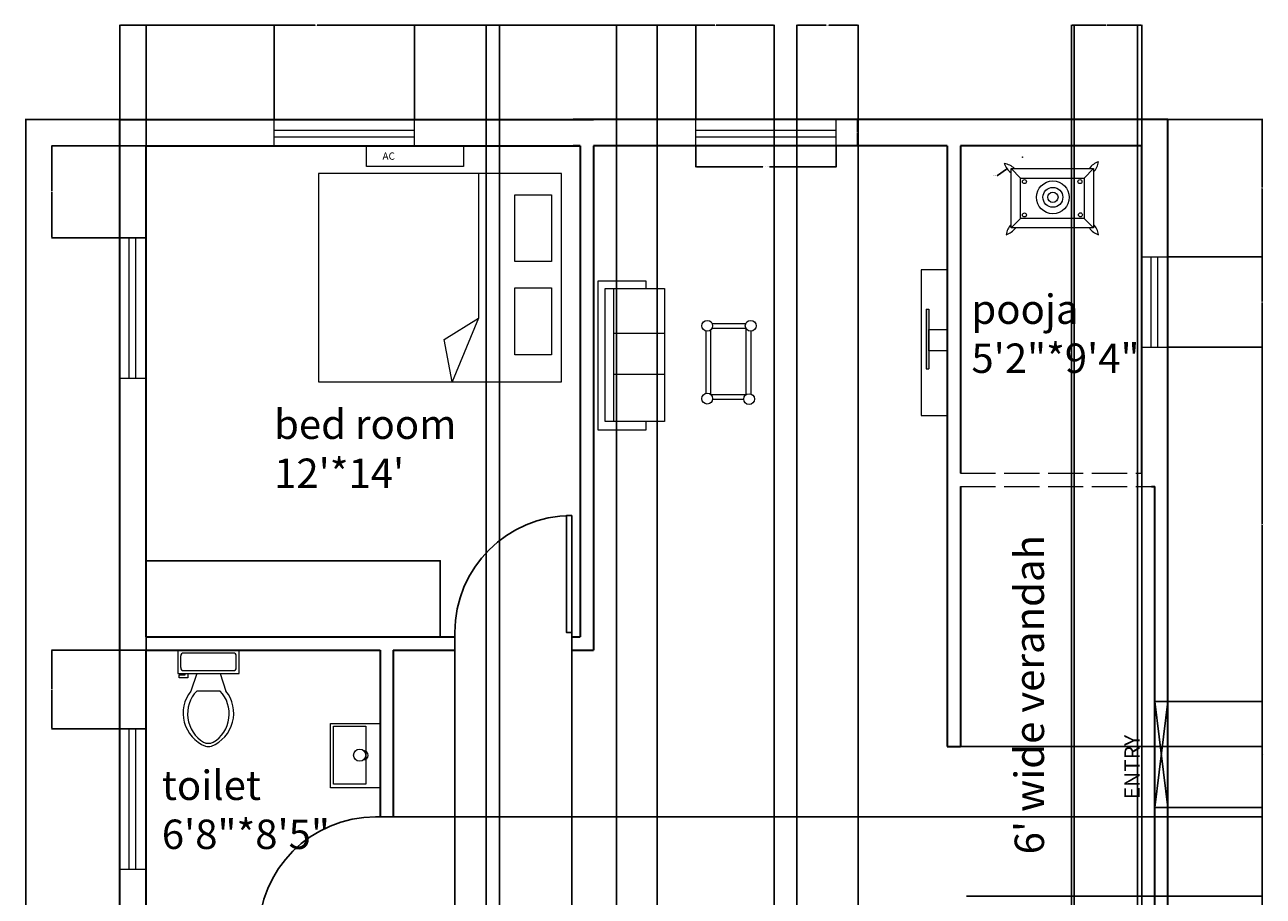
# Model space of a CAD drawing. Units: inches. Extents: x 2187 to 2611, y 763 to 1433.
# Tile 3 of 3: x 2187 to 2611, y 1135 to 1433. Entities that reach past the tile are written whole.
import ezdxf

# ---------------------------------------------------------------- set-up
doc = ezdxf.new("R2010")
doc.units = ezdxf.units.IN
doc.linetypes.add('ACAD_ISO02W100', pattern=[15, 12, -3])
for name, color, linetype, lineweight in [('A-ANNO-DIMS', 2, 'Continuous', 18), ('A-ANNO-TEXT', 7, 'Continuous', 18), ('A-AREA-IDEN', 7, 'Continuous', 18), ('A-FLOR-CASE', 82, 'Continuous', 25), ('A-FLOR-FIXT', 82, 'Continuous', 18), ('A-FURN-PATT', 82, 'Continuous', 13), ('A-WALL', 7, 'Continuous', 35), ('A-WALL-OVHD', 7, 'ACAD_ISO02W100', 18), ('DOOR', 130, 'Continuous', 25), ('FURNITURE', 82, 'Continuous', 18), ('M-HVAC-EQPM', 82, 'Continuous', 18), ('WINDOW', 50, 'Continuous', 20)]:
    doc.layers.add(name, color=color, linetype=linetype, lineweight=lineweight)
doc.styles.get("Standard").update_dxf_attribs({"font": 'arial.ttf'})
doc.dimstyles.get("Standard").update_dxf_attribs({"dimtxt": 0.18, "dimasz": 0.18, "dimexe": 0.18, "dimexo": 0.0625, "dimgap": 0.09, "dimtad": 0, "dimtih": 1, "dimtoh": 1, "dimdec": 4, "dimzin": 0, "dimdsep": 46, "dimtxsty": 'Standard', "dimcen": 0.09, "dimadec": 0, "dimazin": 0, "dimtfac": 1, "dimtdec": 4, "dimtofl": 0, "dimtmove": 0, "dimatfit": 3, "dimfxl": 1, "dimtolj": 1, "dimtzin": 0, "dimarcsym": 0})

# ---------------------------------------------------------------- blocks, each defined once
blk = doc.blocks.new('*U2')
for p, q in [((0, 0), (0, -6)), ((40, 0), (40, -6))]:
    blk.add_line(p, q)
blk.add_lwpolyline([(0, 0), (0, 40), (1.75, 40), (1.75, 0)], close=True)
blk.add_arc((0, 0), 40, 0, 90)
blk = doc.blocks.new('*U4')
for p, q in [((9.5, -6), (9.5, -2)), ((-8, -8.5), (-8, -8)), ((-7, -8), (-7, -9.5)), ((-4, -8), (-6, -14)), ((4, -8), (6, -14)), ((-10, -8.5), (-8, -8.5)), ((-10, -9.5), (-10, -8.5)), ((-7, -9.5), (-10, -9.5)), ((4, -14), (-4, -14))]:
    blk.add_line(p, q)
blk.add_lwpolyline([(10.5, -8), (10.5, 0), (-10.5, 0), (-10.5, -8)], close=True)
for points in [[(-9.5, -2), (-9.5, -6)], [(8.5, -1), (-8.5, -1)], [(-8.5, -7), (8.5, -7)]]:
    blk.add_lwpolyline(points)
for centre, radius, start, end in [((-8.62, -1.88), 0.884, 81.8699, 188.1301), ((8.62, -1.88), 0.884, 351.8699, 98.1301), ((-8.62, -6.12), 0.884, 171.8699, 278.1301), ((8.62, -6.12), 0.884, 261.8699, 8.1301), ((3.52, -21.58), 12.17, 141.4691, 247.9714), ((4.2, -21.82), 11.33, 136.3677, 238.9468), ((-3.52, -21.58), 12.17, 292.0284, 38.5307), ((-4.2, -21.82), 11.33, 301.053, 43.6321), ((0, -27.88), 4, 245.7318, 294.2682), ((0, -29), 4, 254.8605, 285.1395)]:
    blk.add_arc(centre, radius, start, end)
blk = doc.blocks.new('BED-DOUBLE')
for p, q in [((54.72, 71.29), (54.72, 21.8)), ((42.94, 14.53), (54.72, 21.8)), ((54.72, 21.8), (45.71, 0)), ((45.71, 0), (42.94, 14.53))]:
    blk.add_line(p, q)
for points in [[(83.12, 71.29), (0, 71.29), (0, 0), (83.12, 0)], [(67.19, 64.02), (79.65, 64.02), (79.65, 41.18), (67.19, 41.18)], [(67.19, 32.18), (79.65, 32.18), (79.65, 9.34), (67.19, 9.34)]]:
    blk.add_lwpolyline(points, close=True)
blk = doc.blocks.new('WIN-48IN')
for p, q in [((0, 0), (0, 9)), ((48, 0), (48, 9)), ((0, 5.37), (48, 5.37)), ((0, 3.09), (48, 3.09))]:
    blk.add_line(p, q)
blk = doc.blocks.new('*D8')
at = {"layer": 'A-ANNO-DIMS', "color": 0, "lineweight": -2, "transparency": 16777216}
for p, q in [((2416.82, 1391.9), (2416.82, 1384.58)), ((2464.82, 1391.9), (2464.82, 1384.58)), ((2417, 1384.76), (2439.7, 1384.76)), ((2464.64, 1384.76), (2441.94, 1384.76))]:
    blk.add_line(p, q, dxfattribs=at)
at = {"layer": 'A-ANNO-DIMS', "color": 0, "lineweight": 100, "transparency": 16777216}
for points in [[(2417, 1384.79), (2417, 1384.73), (2416.82, 1384.76)], [(2464.64, 1384.79), (2464.64, 1384.73), (2464.82, 1384.76)]]:
    blk.add_solid(points, dxfattribs=at)
at = {"layer": 'Defpoints', "color": 0, "lineweight": 100, "transparency": 16777216}
for p in [(2416.82, 1391.96), (2464.82, 1391.96), (2464.82, 1384.76)]:
    blk.add_point(p, dxfattribs=at)
at = {"layer": 'A-ANNO-DIMS', "color": 0, "transparency": 16777216, "insert": (2440.82, 1384.76), "char_height": 0.18, "attachment_point": 5}
blk.add_mtext('\\A1;WINDOW 48 TYP.', dxfattribs=at)
blk = doc.blocks.new('*D9')
at = {"layer": 'A-ANNO-DIMS', "color": 0, "lineweight": -2, "transparency": 16777216}
for p, q in [((2464.88, 1400.96), (2472.2, 1400.96)), ((2472.02, 1400.78), (2472.02, 1396.64)), ((2472.02, 1392.14), (2472.02, 1396.28)), ((2464.88, 1391.96), (2472.2, 1391.96))]:
    blk.add_line(p, q, dxfattribs=at)
at = {"layer": 'A-ANNO-DIMS', "color": 0, "lineweight": 100, "transparency": 16777216}
for points in [[(2471.99, 1400.78), (2472.05, 1400.78), (2472.02, 1400.96)], [(2471.99, 1392.14), (2472.05, 1392.14), (2472.02, 1391.96)]]:
    blk.add_solid(points, dxfattribs=at)
at = {"layer": 'Defpoints', "color": 0, "lineweight": 100, "transparency": 16777216}
for p in [(2464.82, 1400.96), (2472.02, 1400.96), (2464.82, 1391.96)]:
    blk.add_point(p, dxfattribs=at)
at = {"layer": 'A-ANNO-DIMS', "color": 0, "transparency": 16777216, "insert": (2472.02, 1396.46), "char_height": 0.18, "attachment_point": 5}
blk.add_mtext('\\A1;9 TYP.', dxfattribs=at)
blk = doc.blocks.new('*D15')
at = {"layer": 'A-ANNO-DIMS', "color": 0, "lineweight": -2, "transparency": 16777216}
for p, q in [((2219.71, 1400.96), (2187.39, 1400.96)), ((2187.57, 1400.78), (2187.57, 1120.06)), ((2187.57, 838.97), (2187.57, 1119.7)), ((2219.71, 838.79), (2187.39, 838.79))]:
    blk.add_line(p, q, dxfattribs=at)
at = {"layer": 'A-ANNO-DIMS', "color": 0, "lineweight": 100, "transparency": 16777216}
for points in [[(2187.54, 1400.78), (2187.6, 1400.78), (2187.57, 1400.96)], [(2187.54, 838.97), (2187.6, 838.97), (2187.57, 838.79)]]:
    blk.add_solid(points, dxfattribs=at)
at = {"layer": 'Defpoints', "color": 0, "lineweight": 100, "transparency": 16777216}
for p in [(2187.57, 1400.96), (2219.77, 1400.96), (2219.77, 838.79)]:
    blk.add_point(p, dxfattribs=at)
at = {"layer": 'A-ANNO-DIMS', "color": 0, "transparency": 16777216, "insert": (2187.57, 1119.88), "char_height": 0.18, "attachment_point": 5}
blk.add_mtext('\\A1;562.2', dxfattribs=at)
blk = doc.blocks.new('*D16')
at = {"layer": 'A-ANNO-DIMS', "color": 0, "lineweight": -2, "transparency": 16777216}
for p, q in [((2219.77, 1401.02), (2219.77, 1433.34)), ((2219.95, 1433.16), (2245.76, 1433.16)), ((2272.37, 1433.16), (2246.55, 1433.16)), ((2272.55, 1401.02), (2272.55, 1433.34))]:
    blk.add_line(p, q, dxfattribs=at)
at = {"layer": 'A-ANNO-DIMS', "color": 0, "lineweight": 100, "transparency": 16777216}
for points in [[(2219.95, 1433.19), (2219.95, 1433.13), (2219.77, 1433.16)], [(2272.37, 1433.19), (2272.37, 1433.13), (2272.55, 1433.16)]]:
    blk.add_solid(points, dxfattribs=at)
at = {"layer": 'Defpoints', "color": 0, "lineweight": 100, "transparency": 16777216}
for p in [(2272.55, 1433.16), (2219.77, 1400.96), (2272.55, 1400.96)]:
    blk.add_point(p, dxfattribs=at)
at = {"layer": 'A-ANNO-DIMS', "color": 0, "transparency": 16777216, "insert": (2246.16, 1433.16), "char_height": 0.18, "attachment_point": 5}
blk.add_mtext('\\A1;52.78', dxfattribs=at)
blk = doc.blocks.new('*D17')
at = {"layer": 'A-ANNO-DIMS', "color": 0, "lineweight": -2, "transparency": 16777216}
for p, q in [((2320.55, 1401.02), (2320.55, 1433.34)), ((2320.73, 1433.16), (2368.29, 1433.16)), ((2416.64, 1433.16), (2369.08, 1433.16)), ((2416.82, 1401.02), (2416.82, 1433.34))]:
    blk.add_line(p, q, dxfattribs=at)
at = {"layer": 'A-ANNO-DIMS', "color": 0, "lineweight": 100, "transparency": 16777216}
for points in [[(2320.73, 1433.19), (2320.73, 1433.13), (2320.55, 1433.16)], [(2416.64, 1433.19), (2416.64, 1433.13), (2416.82, 1433.16)]]:
    blk.add_solid(points, dxfattribs=at)
at = {"layer": 'Defpoints', "color": 0, "lineweight": 100, "transparency": 16777216}
for p in [(2416.82, 1433.16), (2320.55, 1400.96), (2416.82, 1400.96)]:
    blk.add_point(p, dxfattribs=at)
at = {"layer": 'A-ANNO-DIMS', "color": 0, "transparency": 16777216, "insert": (2368.68, 1433.16), "char_height": 0.18, "attachment_point": 5}
blk.add_mtext('\\A1;96.28', dxfattribs=at)
blk = doc.blocks.new('*D18')
at = {"layer": 'A-ANNO-DIMS', "color": 0, "lineweight": -2, "transparency": 16777216}
for p, q in [((2228.71, 1391.96), (2196.39, 1391.96)), ((2196.57, 1391.78), (2196.57, 1376.39)), ((2196.57, 1360.64), (2196.57, 1376.03)), ((2228.71, 1360.46), (2196.39, 1360.46))]:
    blk.add_line(p, q, dxfattribs=at)
at = {"layer": 'A-ANNO-DIMS', "color": 0, "lineweight": 100, "transparency": 16777216}
for points in [[(2196.54, 1391.78), (2196.6, 1391.78), (2196.57, 1391.96)], [(2196.54, 1360.64), (2196.6, 1360.64), (2196.57, 1360.46)]]:
    blk.add_solid(points, dxfattribs=at)
at = {"layer": 'Defpoints', "color": 0, "lineweight": 100, "transparency": 16777216}
for p in [(2196.57, 1391.96), (2228.77, 1391.96), (2228.77, 1360.46)]:
    blk.add_point(p, dxfattribs=at)
at = {"layer": 'A-ANNO-DIMS', "color": 0, "transparency": 16777216, "insert": (2196.57, 1376.21), "char_height": 0.18, "attachment_point": 5}
blk.add_mtext('\\A1;31.5', dxfattribs=at)
blk = doc.blocks.new('*D19')
at = {"layer": 'A-ANNO-DIMS', "color": 0, "lineweight": -2, "transparency": 16777216}
for p, q in [((2228.71, 1219.46), (2196.39, 1219.46)), ((2196.57, 1219.28), (2196.57, 1206.18)), ((2196.57, 1192.72), (2196.57, 1205.82)), ((2228.71, 1192.54), (2196.39, 1192.54))]:
    blk.add_line(p, q, dxfattribs=at)
at = {"layer": 'A-ANNO-DIMS', "color": 0, "lineweight": 100, "transparency": 16777216}
for points in [[(2196.54, 1219.28), (2196.6, 1219.28), (2196.57, 1219.46)], [(2196.54, 1192.72), (2196.6, 1192.72), (2196.57, 1192.54)]]:
    blk.add_solid(points, dxfattribs=at)
at = {"layer": 'Defpoints', "color": 0, "lineweight": 100, "transparency": 16777216}
for p in [(2196.57, 1219.46), (2228.77, 1219.46), (2228.77, 1192.54)]:
    blk.add_point(p, dxfattribs=at)
at = {"layer": 'A-ANNO-DIMS', "color": 0, "transparency": 16777216, "insert": (2196.57, 1206), "char_height": 0.18, "attachment_point": 5}
blk.add_mtext('\\A1;26.923', dxfattribs=at)
blk = doc.blocks.new('*D22')
at = {"layer": 'A-ANNO-DIMS', "color": 0, "lineweight": -2, "transparency": 16777216}
for p, q in [((2578.33, 1400.96), (2610.65, 1400.96)), ((2610.47, 1400.78), (2610.47, 1377.65)), ((2610.47, 1354.16), (2610.47, 1377.29)), ((2578.33, 1353.98), (2610.65, 1353.98))]:
    blk.add_line(p, q, dxfattribs=at)
at = {"layer": 'A-ANNO-DIMS', "color": 0, "lineweight": 100, "transparency": 16777216}
for points in [[(2610.44, 1400.78), (2610.5, 1400.78), (2610.47, 1400.96)], [(2610.44, 1354.16), (2610.5, 1354.16), (2610.47, 1353.98)]]:
    blk.add_solid(points, dxfattribs=at)
at = {"layer": 'Defpoints', "color": 0, "lineweight": 100, "transparency": 16777216}
for p in [(2578.27, 1400.96), (2610.47, 1400.96), (2578.27, 1353.98)]:
    blk.add_point(p, dxfattribs=at)
at = {"layer": 'A-ANNO-DIMS', "color": 0, "transparency": 16777216, "insert": (2610.47, 1377.47), "char_height": 0.18, "attachment_point": 5}
blk.add_mtext('\\A1;46.98', dxfattribs=at)
blk = doc.blocks.new('*D23')
at = {"layer": 'A-ANNO-DIMS', "color": 0, "lineweight": -2, "transparency": 16777216}
for p, q in [((2578.33, 1353.98), (2610.65, 1353.98)), ((2610.47, 1353.8), (2610.47, 1338.7)), ((2610.47, 1323.23), (2610.47, 1338.33)), ((2578.33, 1323.05), (2610.65, 1323.05))]:
    blk.add_line(p, q, dxfattribs=at)
at = {"layer": 'A-ANNO-DIMS', "color": 0, "lineweight": 100, "transparency": 16777216}
for points in [[(2610.44, 1353.8), (2610.5, 1353.8), (2610.47, 1353.98)], [(2610.44, 1323.23), (2610.5, 1323.23), (2610.47, 1323.05)]]:
    blk.add_solid(points, dxfattribs=at)
at = {"layer": 'Defpoints', "color": 0, "lineweight": 100, "transparency": 16777216}
for p in [(2578.27, 1353.98), (2610.47, 1353.98), (2578.27, 1323.05)]:
    blk.add_point(p, dxfattribs=at)
at = {"layer": 'A-ANNO-DIMS', "color": 0, "transparency": 16777216, "insert": (2610.47, 1338.51), "char_height": 0.18, "attachment_point": 5}
blk.add_mtext('\\A1;30.93', dxfattribs=at)
blk = doc.blocks.new('*D24')
at = {"layer": 'A-ANNO-DIMS', "color": 0, "lineweight": -2, "transparency": 16777216}
for p, q in [((2578.33, 1323.05), (2610.65, 1323.05)), ((2610.47, 1322.87), (2610.47, 1262.64)), ((2610.47, 1202.06), (2610.47, 1262.28)), ((2578.33, 1201.88), (2610.65, 1201.88))]:
    blk.add_line(p, q, dxfattribs=at)
at = {"layer": 'A-ANNO-DIMS', "color": 0, "lineweight": 100, "transparency": 16777216}
for points in [[(2610.44, 1322.87), (2610.5, 1322.87), (2610.47, 1323.05)], [(2610.44, 1202.06), (2610.5, 1202.06), (2610.47, 1201.88)]]:
    blk.add_solid(points, dxfattribs=at)
at = {"layer": 'Defpoints', "color": 0, "lineweight": 100, "transparency": 16777216}
for p in [(2578.27, 1323.05), (2610.47, 1323.05), (2578.27, 1201.88)]:
    blk.add_point(p, dxfattribs=at)
at = {"layer": 'A-ANNO-DIMS', "color": 0, "transparency": 16777216, "insert": (2610.47, 1262.46), "char_height": 0.18, "attachment_point": 5}
blk.add_mtext('\\A1;121.17', dxfattribs=at)
blk = doc.blocks.new('*D25')
at = {"layer": 'A-ANNO-DIMS', "color": 0, "lineweight": -2, "transparency": 16777216}
for p, q in [((2578.33, 1201.88), (2610.65, 1201.88)), ((2610.47, 1201.7), (2610.47, 1183.93)), ((2610.47, 1165.8), (2610.47, 1183.57)), ((2578.33, 1165.62), (2610.65, 1165.62))]:
    blk.add_line(p, q, dxfattribs=at)
at = {"layer": 'A-ANNO-DIMS', "color": 0, "lineweight": 100, "transparency": 16777216}
for points in [[(2610.44, 1201.7), (2610.5, 1201.7), (2610.47, 1201.88)], [(2610.44, 1165.8), (2610.5, 1165.8), (2610.47, 1165.62)]]:
    blk.add_solid(points, dxfattribs=at)
at = {"layer": 'Defpoints', "color": 0, "lineweight": 100, "transparency": 16777216}
for p in [(2578.27, 1201.88), (2610.47, 1201.88), (2578.27, 1165.62)]:
    blk.add_point(p, dxfattribs=at)
at = {"layer": 'A-ANNO-DIMS', "color": 0, "transparency": 16777216, "insert": (2610.47, 1183.75), "char_height": 0.18, "attachment_point": 5}
blk.add_mtext('\\A1;36.256', dxfattribs=at)
blk = doc.blocks.new('*D26')
at = {"layer": 'A-ANNO-DIMS', "color": 0, "lineweight": -2, "transparency": 16777216}
for p, q in [((2578.33, 1165.62), (2610.65, 1165.62)), ((2610.47, 1165.44), (2610.47, 1108.31)), ((2610.47, 1050.81), (2610.47, 1107.94)), ((2578.33, 1050.63), (2610.65, 1050.63))]:
    blk.add_line(p, q, dxfattribs=at)
at = {"layer": 'A-ANNO-DIMS', "color": 0, "lineweight": 100, "transparency": 16777216}
for points in [[(2610.44, 1165.44), (2610.5, 1165.44), (2610.47, 1165.62)], [(2610.44, 1050.81), (2610.5, 1050.81), (2610.47, 1050.63)]]:
    blk.add_solid(points, dxfattribs=at)
at = {"layer": 'Defpoints', "color": 0, "lineweight": 100, "transparency": 16777216}
for p in [(2578.27, 1165.62), (2610.47, 1165.62), (2578.27, 1050.63)]:
    blk.add_point(p, dxfattribs=at)
at = {"layer": 'A-ANNO-DIMS', "color": 0, "transparency": 16777216, "insert": (2610.47, 1108.13), "char_height": 0.18, "attachment_point": 5}
blk.add_mtext('\\A1;114.99', dxfattribs=at)
blk = doc.blocks.new('*D28')
at = {"layer": 'A-ANNO-DIMS', "color": 0, "lineweight": -2, "transparency": 16777216}
for p, q in [((2349.61, 1016.11), (2349.61, 1433.34)), ((2349.79, 1433.16), (2369.39, 1433.16)), ((2389.43, 1433.16), (2369.83, 1433.16)), ((2389.61, 1016.11), (2389.61, 1433.34))]:
    blk.add_line(p, q, dxfattribs=at)
at = {"layer": 'A-ANNO-DIMS', "color": 0, "lineweight": 100, "transparency": 16777216}
for points in [[(2349.79, 1433.19), (2349.79, 1433.13), (2349.61, 1433.16)], [(2389.43, 1433.19), (2389.43, 1433.13), (2389.61, 1433.16)]]:
    blk.add_solid(points, dxfattribs=at)
at = {"layer": 'Defpoints', "color": 0, "lineweight": 100, "transparency": 16777216}
for p in [(2389.61, 1433.16), (2349.61, 1016.04), (2389.61, 1016.04)]:
    blk.add_point(p, dxfattribs=at)
at = {"layer": 'A-ANNO-DIMS', "color": 0, "transparency": 16777216, "insert": (2369.61, 1433.16), "char_height": 0.18, "attachment_point": 5}
blk.add_mtext('\\A1;40', dxfattribs=at)
blk = doc.blocks.new('*D30')
at = {"layer": 'A-ANNO-DIMS', "color": 0, "lineweight": -2, "transparency": 16777216}
for p, q in [((2334.33, 1219.4), (2334.33, 806.41)), ((2374.33, 1219.4), (2374.33, 806.41)), ((2334.51, 806.59), (2354.11, 806.59)), ((2374.15, 806.59), (2354.56, 806.59))]:
    blk.add_line(p, q, dxfattribs=at)
at = {"layer": 'A-ANNO-DIMS', "color": 0, "lineweight": 100, "transparency": 16777216}
for points in [[(2334.51, 806.62), (2334.51, 806.56), (2334.33, 806.59)], [(2374.15, 806.62), (2374.15, 806.56), (2374.33, 806.59)]]:
    blk.add_solid(points, dxfattribs=at)
at = {"layer": 'Defpoints', "color": 0, "lineweight": 100, "transparency": 16777216}
for p in [(2334.33, 1219.46), (2374.33, 1219.46), (2374.33, 806.59)]:
    blk.add_point(p, dxfattribs=at)
at = {"layer": 'A-ANNO-DIMS', "color": 0, "transparency": 16777216, "insert": (2354.33, 806.59), "char_height": 0.18, "attachment_point": 5}
blk.add_mtext('\\A1;40', dxfattribs=at)
blk = doc.blocks.new('*D31')
at = {"layer": 'A-ANNO-DIMS', "color": 0, "lineweight": -2, "transparency": 16777216}
for p, q in [((2313.33, 1162.4), (2610.65, 1162.4)), ((2610.47, 1162.22), (2610.47, 1142.58)), ((2610.47, 1122.58), (2610.47, 1142.22)), ((2313.33, 1122.4), (2610.65, 1122.4))]:
    blk.add_line(p, q, dxfattribs=at)
at = {"layer": 'A-ANNO-DIMS', "color": 0, "lineweight": 100, "transparency": 16777216}
for points in [[(2610.44, 1162.22), (2610.5, 1162.22), (2610.47, 1162.4)], [(2610.44, 1122.58), (2610.5, 1122.58), (2610.47, 1122.4)]]:
    blk.add_solid(points, dxfattribs=at)
at = {"layer": 'Defpoints', "color": 0, "lineweight": 100, "transparency": 16777216}
for p in [(2313.27, 1162.4), (2610.47, 1162.4), (2313.27, 1122.4)]:
    blk.add_point(p, dxfattribs=at)
at = {"layer": 'A-ANNO-DIMS', "color": 0, "transparency": 16777216, "insert": (2610.47, 1142.4), "char_height": 0.18, "attachment_point": 5}
blk.add_mtext('\\A1;40', dxfattribs=at)
blk = doc.blocks.new('*D32')
at = {"layer": 'A-ANNO-DIMS', "color": 0, "lineweight": -2, "transparency": 16777216}
for p, q in [((2507.33, 1186.47), (2610.65, 1186.47)), ((2610.47, 1186.29), (2610.47, 1161.06)), ((2610.47, 1135.46), (2610.47, 1160.69)), ((2509.33, 1135.28), (2610.65, 1135.28))]:
    blk.add_line(p, q, dxfattribs=at)
at = {"layer": 'A-ANNO-DIMS', "color": 0, "lineweight": 100, "transparency": 16777216}
for points in [[(2610.44, 1186.29), (2610.5, 1186.29), (2610.47, 1186.47)], [(2610.44, 1135.46), (2610.5, 1135.46), (2610.47, 1135.28)]]:
    blk.add_solid(points, dxfattribs=at)
at = {"layer": 'Defpoints', "color": 0, "lineweight": 100, "transparency": 16777216}
for p in [(2507.27, 1186.47), (2610.47, 1186.47), (2509.27, 1135.28)]:
    blk.add_point(p, dxfattribs=at)
at = {"layer": 'A-ANNO-DIMS', "color": 0, "transparency": 16777216, "insert": (2610.47, 1160.88), "char_height": 0.18, "attachment_point": 5}
blk.add_mtext('\\A1;51.2', dxfattribs=at)
blk = doc.blocks.new('*D33')
at = {"layer": 'A-ANNO-DIMS', "color": 0, "lineweight": -2, "transparency": 16777216}
for p, q in [((2545.27, 941.86), (2545.27, 1433.34)), ((2545.45, 1433.16), (2557.05, 1433.16)), ((2569.09, 1433.16), (2557.49, 1433.16)), ((2569.27, 941.86), (2569.27, 1433.34))]:
    blk.add_line(p, q, dxfattribs=at)
at = {"layer": 'A-ANNO-DIMS', "color": 0, "lineweight": 100, "transparency": 16777216}
for points in [[(2545.45, 1433.19), (2545.45, 1433.13), (2545.27, 1433.16)], [(2569.09, 1433.19), (2569.09, 1433.13), (2569.27, 1433.16)]]:
    blk.add_solid(points, dxfattribs=at)
at = {"layer": 'Defpoints', "color": 0, "lineweight": 100, "transparency": 16777216}
for p in [(2569.27, 1433.16), (2545.27, 941.79), (2569.27, 941.79)]:
    blk.add_point(p, dxfattribs=at)
at = {"layer": 'A-ANNO-DIMS', "color": 0, "transparency": 16777216, "insert": (2557.27, 1433.16), "char_height": 0.18, "attachment_point": 5}
blk.add_mtext('\\A1;24', dxfattribs=at)
blk = doc.blocks.new('*D36')
at = {"layer": 'A-ANNO-DIMS', "color": 0, "lineweight": -2, "transparency": 16777216}
for p, q in [((2403.54, 946.36), (2403.54, 1433.34)), ((2403.72, 1433.16), (2423.32, 1433.16)), ((2443.36, 1433.16), (2423.76, 1433.16)), ((2443.54, 946.36), (2443.54, 1433.34))]:
    blk.add_line(p, q, dxfattribs=at)
at = {"layer": 'A-ANNO-DIMS', "color": 0, "lineweight": 100, "transparency": 16777216}
for points in [[(2403.72, 1433.19), (2403.72, 1433.13), (2403.54, 1433.16)], [(2443.36, 1433.19), (2443.36, 1433.13), (2443.54, 1433.16)]]:
    blk.add_solid(points, dxfattribs=at)
at = {"layer": 'Defpoints', "color": 0, "lineweight": 100, "transparency": 16777216}
for p in [(2443.54, 1433.16), (2403.54, 946.29), (2443.54, 946.29)]:
    blk.add_point(p, dxfattribs=at)
at = {"layer": 'A-ANNO-DIMS', "color": 0, "transparency": 16777216, "insert": (2423.54, 1433.16), "char_height": 0.18, "attachment_point": 5}
blk.add_mtext('\\A1;40', dxfattribs=at)
blk = doc.blocks.new('*D40')
at = {"layer": 'A-ANNO-DIMS', "color": 0, "lineweight": -2, "transparency": 16777216}
for p, q in [((2451.33, 870.16), (2451.33, 1433.34)), ((2451.51, 1433.16), (2461.34, 1433.16)), ((2472.1, 1433.16), (2462.27, 1433.16)), ((2472.28, 870.16), (2472.28, 1433.34))]:
    blk.add_line(p, q, dxfattribs=at)
at = {"layer": 'A-ANNO-DIMS', "color": 0, "lineweight": 100, "transparency": 16777216}
for points in [[(2451.51, 1433.19), (2451.51, 1433.13), (2451.33, 1433.16)], [(2472.1, 1433.19), (2472.1, 1433.13), (2472.28, 1433.16)]]:
    blk.add_solid(points, dxfattribs=at)
at = {"layer": 'Defpoints', "color": 0, "lineweight": 100, "transparency": 16777216}
for p in [(2472.28, 1433.16), (2451.33, 870.1), (2472.28, 870.1)]:
    blk.add_point(p, dxfattribs=at)
at = {"layer": 'A-ANNO-DIMS', "color": 0, "transparency": 16777216, "insert": (2461.81, 1433.16), "char_height": 0.18, "attachment_point": 5}
blk.add_mtext('\\A1;20.953', dxfattribs=at)
blk = doc.blocks.new('*D42')
at = {"layer": 'A-ANNO-DIMS', "color": 0, "lineweight": -2, "transparency": 16777216}
for p, q in [((2546.19, 933.93), (2546.19, 1433.34)), ((2546.37, 1433.16), (2556.61, 1433.16)), ((2567.64, 1433.16), (2557.4, 1433.16)), ((2567.82, 933.93), (2567.82, 1433.34))]:
    blk.add_line(p, q, dxfattribs=at)
at = {"layer": 'A-ANNO-DIMS', "color": 0, "lineweight": 100, "transparency": 16777216}
for points in [[(2546.37, 1433.19), (2546.37, 1433.13), (2546.19, 1433.16)], [(2567.64, 1433.19), (2567.64, 1433.13), (2567.82, 1433.16)]]:
    blk.add_solid(points, dxfattribs=at)
at = {"layer": 'Defpoints', "color": 0, "lineweight": 100, "transparency": 16777216}
for p in [(2567.82, 1433.16), (2546.19, 933.87), (2567.82, 933.87)]:
    blk.add_point(p, dxfattribs=at)
at = {"layer": 'A-ANNO-DIMS', "color": 0, "transparency": 16777216, "insert": (2557.01, 1433.16), "char_height": 0.18, "attachment_point": 5}
blk.add_mtext('\\A1;21.63', dxfattribs=at)
blk = doc.blocks.new('*D44')
at = {"layer": 'A-ANNO-DIMS', "color": 0, "lineweight": -2, "transparency": 16777216}
for p, q in [((2228.77, 1118.52), (2228.77, 1433.34)), ((2228.95, 1433.16), (2286.53, 1433.16)), ((2344.89, 1433.16), (2287.3, 1433.16)), ((2345.07, 1118.52), (2345.07, 1433.34))]:
    blk.add_line(p, q, dxfattribs=at)
at = {"layer": 'A-ANNO-DIMS', "color": 0, "lineweight": 100, "transparency": 16777216}
for points in [[(2228.95, 1433.19), (2228.95, 1433.13), (2228.77, 1433.16)], [(2344.89, 1433.19), (2344.89, 1433.13), (2345.07, 1433.16)]]:
    blk.add_solid(points, dxfattribs=at)
at = {"layer": 'Defpoints', "color": 0, "lineweight": 100, "transparency": 16777216}
for p in [(2345.07, 1433.16), (2228.77, 1118.46), (2345.07, 1118.46)]:
    blk.add_point(p, dxfattribs=at)
at = {"layer": 'A-ANNO-DIMS', "color": 0, "transparency": 16777216, "insert": (2286.92, 1433.16), "char_height": 0.18, "attachment_point": 5}
blk.add_mtext('\\A1;116.3', dxfattribs=at)
blk = doc.blocks.new('*D50')
at = {"layer": 'A-ANNO-DIMS', "color": 0, "lineweight": -2, "transparency": 16777216}
for p, q in [((2528.47, 1388.04), (2528.65, 1388.04)), ((2528.56, 1387.95), (2528.56, 1388.13)), ((2519.83, 1381.75), (2520.01, 1381.75)), ((2520.01, 1381.75), (2523.07, 1384))]:
    blk.add_line(p, q, dxfattribs=at)
at = {"layer": 'A-ANNO-DIMS', "color": 0, "lineweight": 100, "transparency": 16777216}
blk.add_solid([(2523.05, 1384.03), (2523.09, 1383.98), (2523.21, 1384.11)], dxfattribs=at)
at = {"layer": 'Defpoints', "color": 0, "lineweight": 100, "transparency": 16777216}
for p in [(2528.56, 1388.04), (2523.21, 1384.11)]:
    blk.add_point(p, dxfattribs=at)
at = {"layer": 'A-ANNO-DIMS', "color": 0, "transparency": 16777216, "insert": (2519.15, 1381.75), "char_height": 0.18, "attachment_point": 5}
blk.add_mtext('\\A1;8X R6.637', dxfattribs=at)

msp = doc.modelspace()

# ---------------------------------------------------------------- hatches: boundary and pattern name
at = {"layer": 'A-FURN-PATT'}
h = msp.add_hatch(color=256, dxfattribs=at)
h.dxf.hatch_style = 1
h.paths.add_polyline_path([(2496.4908, 1336.1236), (2495.5884, 1336.1236), (2495.5884, 1315.6079), (2496.4908, 1315.6079)])

# ---------------------------------------------------------------- linework, layer by layer
at = {"layer": 'A-FLOR-CASE'}
msp.add_lwpolyline([(2329.3717, 1223.9602), (2228.7681, 1223.9602), (2228.7681, 1250.0386), (2329.3717, 1250.0386)], close=True, dxfattribs=at)
at = {"layer": 'A-FLOR-FIXT'}
for points in [[(2308.7681, 1172.3661), (2291.8492, 1172.3661), (2291.8492, 1194.3768), (2308.7681, 1194.3768)], [(2292.8216, 1193.4103), (2303.8896, 1193.4103), (2303.8896, 1173.6488), (2292.8216, 1173.6488)]]:
    msp.add_lwpolyline(points, close=True, dxfattribs=at)
msp.add_circle((2301.803, 1183.5295), 2.0866, dxfattribs=at)
msp.add_arc((2303.1264, 1183.4931), 1.5864, 269.578212, 87.265408, dxfattribs=at)
at = {"layer": 'A-WALL'}
for p, q in [((2219.7681, 1223.9602), (2219.7681, 1400.9602)), ((2219.7681, 1400.9602), (2381.7681, 1400.9602)), ((2578.2681, 1400.9602), (2374.7998, 1400.9602)), ((2578.2681, 1219.2937), (2578.2681, 1400.9602)), ((2228.7681, 1223.9602), (2228.7681, 1391.9602)), ((2228.7681, 1391.9602), (2372.7681, 1391.9602)), ((2372.7681, 1391.9602), (2377.2681, 1391.9602)), ((2377.2681, 1391.9602), (2374.7998, 1391.9602)), ((2377.2681, 1391.9602), (2377.2681, 1223.9602)), ((2381.7681, 1391.9602), (2381.7681, 1219.4602)), ((2502.7681, 1391.9602), (2381.7681, 1391.9602)), ((2502.7681, 1391.9602), (2502.7681, 1275.4602)), ((2569.2681, 1391.9602), (2507.2681, 1391.9602)), ((2569.2681, 1391.9602), (2507.2681, 1391.9602)), ((2507.2681, 1391.9602), (2507.2681, 1279.9602)), ((2569.2681, 1279.9602), (2569.2681, 1391.9602)), ((2502.7681, 1275.4602), (2502.7681, 1186.4745)), ((2507.2681, 1275.4602), (2507.2681, 1186.4745)), ((2572.626, 1275.4602), (2573.7681, 1275.4602)), ((2573.7681, 1075.2937), (2573.7681, 1275.4602)), ((2578.2681, 1075.2937), (2578.2681, 1275.4602)), ((2219.7681, 1118.4602), (2219.7681, 1223.9602)), ((2228.7681, 1223.9602), (2334.3333, 1223.9602)), ((2374.3333, 1223.9602), (2377.2681, 1223.9602)), ((2228.7681, 1118.4602), (2228.7681, 1219.4602)), ((2228.7681, 1219.4602), (2308.7681, 1219.4602)), ((2228.7681, 1219.4602), (2308.7681, 1219.4602)), ((2308.7681, 1219.4602), (2308.7681, 1162.3972)), ((2313.2681, 1219.4602), (2313.2681, 1162.3972)), ((2313.2681, 1219.4602), (2334.3333, 1219.4602)), ((2374.3333, 1219.4602), (2381.7681, 1219.4602)), ((2502.7681, 1186.4745), (2507.2681, 1186.4745))]:
    msp.add_line(p, q, dxfattribs=at)
at = {"layer": 'A-WALL-OVHD'}
for p, q in [((2507.2681, 1279.9602), (2569.2681, 1279.9602)), ((2507.2681, 1275.4602), (2573.7681, 1275.4602))]:
    msp.add_line(p, q, dxfattribs=at)
at = {"layer": 'DOOR'}
for p, q in [((2578.2681, 1201.8762), (2573.7681, 1201.8762)), ((2573.7681, 1165.6205), (2578.2681, 1201.8762)), ((2573.7681, 1201.8762), (2578.2681, 1165.6205)), ((2573.7681, 1165.6205), (2578.2681, 1165.6205))]:
    msp.add_line(p, q, dxfattribs=at)
at = {"layer": 'FURNITURE'}
for p, q in [((2527.8538, 1380.916), (2524.6148, 1384.155)), ((2524.6148, 1384.155), (2552.8254, 1384.155)), ((2552.8254, 1384.155), (2549.5864, 1380.916)), ((2549.5864, 1380.916), (2549.5864, 1367.0846)), ((2524.6148, 1363.8456), (2527.8538, 1367.0846)), ((2549.5864, 1367.0846), (2552.8254, 1363.8456)), ((2552.8254, 1363.8456), (2524.6148, 1363.8456)), ((2399.7715, 1345.5894), (2383.2074, 1345.5894)), ((2383.2074, 1345.5894), (2383.2074, 1294.77)), ((2388.5915, 1343.184), (2388.5915, 1297.6288)), ((2399.7715, 1343.184), (2399.7715, 1345.5894)), ((2495.5884, 1336.1236), (2495.5884, 1315.6079)), ((2495.5884, 1336.1236), (2496.4908, 1336.1236)), ((2496.4908, 1336.1236), (2496.4908, 1315.6079)), ((2388.5915, 1327.8565), (2406.028, 1327.8565)), ((2420.2847, 1328.1984), (2420.2847, 1328.5854)), ((2388.5915, 1313.8839), (2406.028, 1313.8839)), ((2495.5884, 1315.6079), (2496.4908, 1315.6079)), ((2399.7715, 1294.77), (2399.7715, 1297.6288)), ((2383.2074, 1294.77), (2399.7715, 1294.77))]:
    msp.add_line(p, q, dxfattribs=at)
for points in [[(2524.6148, 1384.155), (2552.8254, 1384.155), (2552.8254, 1363.8456), (2524.6148, 1363.8456)], [(2527.8538, 1380.916), (2549.5864, 1380.916), (2549.5864, 1367.0846), (2527.8538, 1367.0846)], [(2502.7681, 1349.5687), (2493.7941, 1349.5687), (2493.7941, 1299.6738), (2502.7681, 1299.6738)], [(2385.752, 1343.184), (2406.028, 1343.184), (2406.028, 1297.6288), (2385.752, 1297.6288)], [(2496.4908, 1329.0995), (2502.7681, 1329.0995), (2502.7681, 1321.7683), (2496.4908, 1321.7683)]]:
    msp.add_lwpolyline(points, close=True, dxfattribs=at)
for points in [[(2422.3425, 1331.1854), (2433.8784, 1331.1854)], [(2420.2847, 1307.2776), (2420.2847, 1328.2421)], [(2421.9458, 1306.8211), (2421.9458, 1329.0419)], [(2422.3142, 1329.5243), (2433.9119, 1329.5243), (2433.9119, 1306.8092)], [(2435.573, 1328.5423), (2435.573, 1307.0647)], [(2433.893, 1306.7954), (2421.9726, 1306.7954)], [(2433.1541, 1305.1343), (2422.4976, 1305.1343)]]:
    msp.add_lwpolyline(points, dxfattribs=at)
for centre, radius in [((2529.1776, 1379.6822), 0.6865), ((2538.9004, 1374.3203), 5.5971), ((2538.9004, 1374.3203), 3.3995), ((2548.1585, 1379.6822), 0.6865), ((2538.9004, 1374.3203), 1.7546), ((2529.1776, 1368.2959), 0.6865), ((2548.3301, 1368.3302), 0.6865), ((2420.6823, 1330.3889), 1.8468), ((2435.5446, 1330.3889), 1.8468), ((2420.6823, 1305.4741), 1.8468), ((2434.9924, 1305.3115), 1.8468)]:
    msp.add_circle(centre, radius, dxfattribs=at)
for centre, start, end in [((2528.5609, 1388.0411), 199.145096, 233.516075), ((2521.273, 1379.3064), 46.934409, 81.173424), ((2556.7115, 1380.2258), 109.145096, 143.516075), ((2547.9768, 1387.5138), 316.934409, 351.173424), ((2529.4634, 1360.483), 136.934409, 171.173424), ((2547.9768, 1360.5187), 8.826576, 43.065591), ((2520.7287, 1367.771), 289.145096, 323.516075), ((2556.7115, 1367.8066), 216.483925, 250.854904)]:
    msp.add_arc(centre, 6.6367, start, end, dxfattribs=at)
at = {"layer": 'M-HVAC-EQPM'}
msp.add_lwpolyline([(2304.1109, 1391.9602), (2337.2656, 1391.9602), (2337.2656, 1384.8209), (2304.1109, 1384.8209)], close=True, dxfattribs=at)
at = {"layer": 'WINDOW'}
for p, q in [((2569.2681, 1353.9807), (2578.2681, 1353.9807)), ((2572.3628, 1353.9807), (2572.3628, 1323.0488)), ((2574.6351, 1353.9807), (2574.6351, 1323.0488)), ((2569.2681, 1323.0488), (2578.2681, 1323.0488))]:
    msp.add_line(p, q, dxfattribs=at)

# ---------------------------------------------------------------- block references
at = {"layer": 'A-FLOR-FIXT'}
msp.add_blockref('*U4', (2250.0791, 1219.4602), dxfattribs=at)
at = {"layer": 'DOOR', "xscale": -1}
msp.add_blockref('*U2', (2374.3333, 1225.4602), dxfattribs=at)
at = {"layer": 'DOOR', "rotation": 90.00000000000003}
msp.add_blockref('*U2', (2307.2681, 1122.3972), dxfattribs=at)
at = {"layer": 'FURNITURE'}
msp.add_blockref('BED-DOUBLE', (2287.7239, 1311.1636), dxfattribs=at)
at = {"layer": 'WINDOW'}
for p in [(2272.5459, 1391.9602), (2416.8218, 1391.9602)]:
    msp.add_blockref('WIN-48IN', p, dxfattribs=at)
at = {"layer": 'WINDOW', "rotation": 270.000000000001}
for p in [(2219.7681, 1360.4602), (2219.7681, 1192.5373)]:
    msp.add_blockref('WIN-48IN', p, dxfattribs=at)

# ---------------------------------------------------------------- texts
at = {"layer": 'A-ANNO-TEXT', "insert": (2309.6041, 1389.6704), "char_height": 2.5, "attachment_point": 1}
msp.add_mtext_dynamic_manual_height_columns('AC', width=7.404151, gutter_width=12.5, heights=[0], dxfattribs=at)
at = {"layer": 'A-ANNO-TEXT', "insert": (2563.3618, 1168.4532), "char_height": 5.24212, "attachment_point": 1, "rotation": 90}
msp.add_mtext_dynamic_manual_height_columns('ENTRY', width=83.616255, gutter_width=26.2106, heights=[0], dxfattribs=at)
at = {"layer": 'A-AREA-IDEN', "char_height": 10.05676, "attachment_point": 1}
for s, insert in [('pooja\\P5\'2"*9\'4"', (2511.0356, 1341.0888)), ("bed room\\P12'*14'", (2272.5448, 1301.7372)), ('toilet\\P6\'8"*8\'5"', (2234.1313, 1178.2554))]:
    msp.add_mtext_dynamic_manual_height_columns(s, width=160.413815, gutter_width=50.2838, heights=[0], dxfattribs=dict(at, insert=insert))
at = {"layer": 'A-AREA-IDEN', "insert": (2525.8168, 1149.5946), "char_height": 10.056757, "attachment_point": 1, "rotation": 90}
msp.add_mtext_dynamic_manual_height_columns("6' wide verandah", width=160.413815, gutter_width=50.2838, heights=[0], dxfattribs=at)

# ---------------------------------------------------------------- dimensions: what is measured, and where the dimension line sits
at = {"layer": 'A-ANNO-DIMS'}
for base, p1, p2, override, picture, middle in [((2272.5459, 1433.1602), (2219.7681, 1400.9602), (2272.5459, 1400.9602), {"dimdec": 2, "dimlfac": 1, "dimrnd": 0, "dimzin": 0, "dimdsep": 46, "dimlunit": 2}, '*D16', (2246.157, 1433.1602)), ((2345.0663, 1433.1602), (2228.7681, 1118.4602), (2345.0663, 1118.4602), {"dimdec": 1, "dimlfac": 1, "dimrnd": 0, "dimzin": 0, "dimdsep": 46, "dimlunit": 2}, '*D44', (2286.9172, 1433.1602)), ((2416.8218, 1433.1602), (2320.5459, 1400.9602), (2416.8218, 1400.9602), {"dimdec": 2, "dimlfac": 1, "dimrnd": 0, "dimzin": 0, "dimdsep": 46, "dimlunit": 2}, '*D17', (2368.6839, 1433.1602)), ((2389.6096, 1433.1602), (2349.6096, 1016.0437), (2389.6096, 1016.0437), {"dimdec": 0, "dimlfac": 1, "dimrnd": 0, "dimzin": 0, "dimdsep": 46, "dimlunit": 2}, '*D28', (2369.6096, 1433.1602)), ((2443.5404, 1433.1602), (2403.5404, 946.2937), (2443.5404, 946.2937), {"dimdec": 0, "dimlfac": 1, "dimrnd": 0, "dimzin": 0, "dimdsep": 46, "dimlunit": 2}, '*D36', (2423.5404, 1433.1602)), ((2472.2814, 1433.1602), (2451.3286, 870.1006), (2472.2814, 870.1006), {"dimdec": 3, "dimlfac": 1, "dimrnd": 0, "dimzin": 0, "dimdsep": 46, "dimlunit": 2}, '*D40', (2461.805, 1433.1602)), ((2569.2681, 1433.1602), (2545.2681, 941.7937), (2569.2681, 941.7937), {"dimdec": 0, "dimlfac": 1, "dimrnd": 0, "dimzin": 0, "dimdsep": 46, "dimlunit": 2}, '*D33', (2557.2681, 1433.1602)), ((2567.8237, 1433.1602), (2546.1934, 933.8683), (2567.8237, 933.8683), {"dimdec": 2, "dimlfac": 1, "dimrnd": 0, "dimzin": 0, "dimdsep": 46, "dimlunit": 2}, '*D42', (2557.0086, 1433.1602)), ((2374.3333, 806.5937), (2334.3333, 1219.4602), (2374.3333, 1219.4602), {"dimdec": 0, "dimlfac": 1, "dimrnd": 0, "dimzin": 0, "dimdsep": 46, "dimlunit": 2}, '*D30', (2354.3333, 806.5937))]:
    dim = msp.add_linear_dim(base=base, p1=p1, p2=p2, dimstyle='Standard', override=override, dxfattribs=at)
    dim.commit()
    dim.dimension.update_dxf_attribs({"geometry": picture, "text_midpoint": middle})
for base, p1, p2, override, picture, middle in [((2187.5681, 1400.9602), (2219.7681, 838.7937), (2219.7681, 1400.9602), {"dimdec": 1, "dimlfac": 1, "dimrnd": 0, "dimzin": 0, "dimdsep": 46, "dimlunit": 2}, '*D15', (2187.5681, 1119.877)), ((2610.4681, 1400.9602), (2578.2681, 1353.9807), (2578.2681, 1400.9602), {"dimdec": 2, "dimlfac": 1, "dimrnd": 0, "dimzin": 0, "dimdsep": 46, "dimlunit": 2}, '*D22', (2610.4681, 1377.4704)), ((2196.5681, 1391.9602), (2228.7681, 1360.4602), (2228.7681, 1391.9602), {"dimdec": 1, "dimlfac": 1, "dimrnd": 0, "dimzin": 0, "dimdsep": 46, "dimlunit": 2}, '*D18', (2196.5681, 1376.2102)), ((2610.4681, 1353.9807), (2578.2681, 1323.0488), (2578.2681, 1353.9807), {"dimdec": 2, "dimlfac": 1, "dimrnd": 0, "dimzin": 0, "dimdsep": 46, "dimlunit": 2}, '*D23', (2610.4681, 1338.5148)), ((2610.4681, 1323.0488), (2578.2681, 1201.8762), (2578.2681, 1323.0488), {"dimdec": 2, "dimlfac": 1, "dimrnd": 0, "dimzin": 0, "dimdsep": 46, "dimlunit": 2}, '*D24', (2610.4681, 1262.4625)), ((2196.5681, 1219.4602), (2228.7681, 1192.5373), (2228.7681, 1219.4602), {"dimdec": 3, "dimlfac": 1, "dimrnd": 0, "dimzin": 0, "dimdsep": 46, "dimlunit": 2}, '*D19', (2196.5681, 1205.9987)), ((2610.4681, 1201.8762), (2578.2681, 1165.6205), (2578.2681, 1201.8762), {"dimdec": 3, "dimlfac": 1, "dimrnd": 0, "dimzin": 0, "dimdsep": 46, "dimlunit": 2}, '*D25', (2610.4681, 1183.7484)), ((2610.4681, 1186.4745), (2509.2681, 1135.278), (2507.2681, 1186.4745), {"dimdec": 1, "dimlfac": 1, "dimrnd": 0, "dimzin": 0, "dimdsep": 46, "dimlunit": 2}, '*D32', (2610.4681, 1160.8762)), ((2610.4681, 1165.6205), (2578.2681, 1050.6332), (2578.2681, 1165.6205), {"dimdec": 2, "dimlfac": 1, "dimrnd": 0, "dimzin": 0, "dimdsep": 46, "dimlunit": 2}, '*D26', (2610.4681, 1108.1268)), ((2610.4681, 1162.3972), (2313.2681, 1122.3972), (2313.2681, 1162.3972), {"dimdec": 0, "dimlfac": 1, "dimrnd": 0, "dimzin": 0, "dimdsep": 46, "dimlunit": 2}, '*D31', (2610.4681, 1142.3972))]:
    dim = msp.add_linear_dim(base=base, p1=p1, p2=p2, angle=90, dimstyle='Standard', override=override, dxfattribs=at)
    dim.commit()
    dim.dimension.update_dxf_attribs({"geometry": picture, "text_midpoint": middle})
dim = msp.add_linear_dim(base=(2472.0218, 1400.9602), p1=(2464.8218, 1391.9602), p2=(2464.8218, 1400.9602), angle=90, text='<> TYP.', dimstyle='Standard', override={"dimdec": 0, "dimlfac": 1, "dimrnd": 0, "dimzin": 0, "dimdsep": 46, "dimlunit": 2}, dxfattribs=at)
dim.commit()
dim.dimension.update_dxf_attribs({"geometry": '*D9', "text_midpoint": (2472.0218, 1396.4602)})
dim = msp.add_linear_dim(base=(2464.8218, 1384.7602), p1=(2416.8218, 1391.9602), p2=(2464.8218, 1391.9602), text='WINDOW <> TYP.', dimstyle='Standard', override={"dimdec": 0, "dimlfac": 1, "dimrnd": 0, "dimzin": 0, "dimdsep": 46, "dimlunit": 2}, dxfattribs=at)
dim.commit()
dim.dimension.update_dxf_attribs({"geometry": '*D8', "text_midpoint": (2440.8218, 1384.7602)})
dim = msp.add_radius_dim(center=(2528.5609, 1388.0411), mpoint=(2523.2143, 1384.1093), text='8X <>', dimstyle='Standard', override={"dimdec": 3, "dimlfac": 1, "dimrnd": 0, "dimzin": 0, "dimdsep": 46, "dimlunit": 2}, dxfattribs=at)
dim.commit()
dim.dimension.update_dxf_attribs({"geometry": '*D50', "text_midpoint": (2519.153, 1381.7501), "dimtype": 164})

doc.saveas('drawing.dxf')
